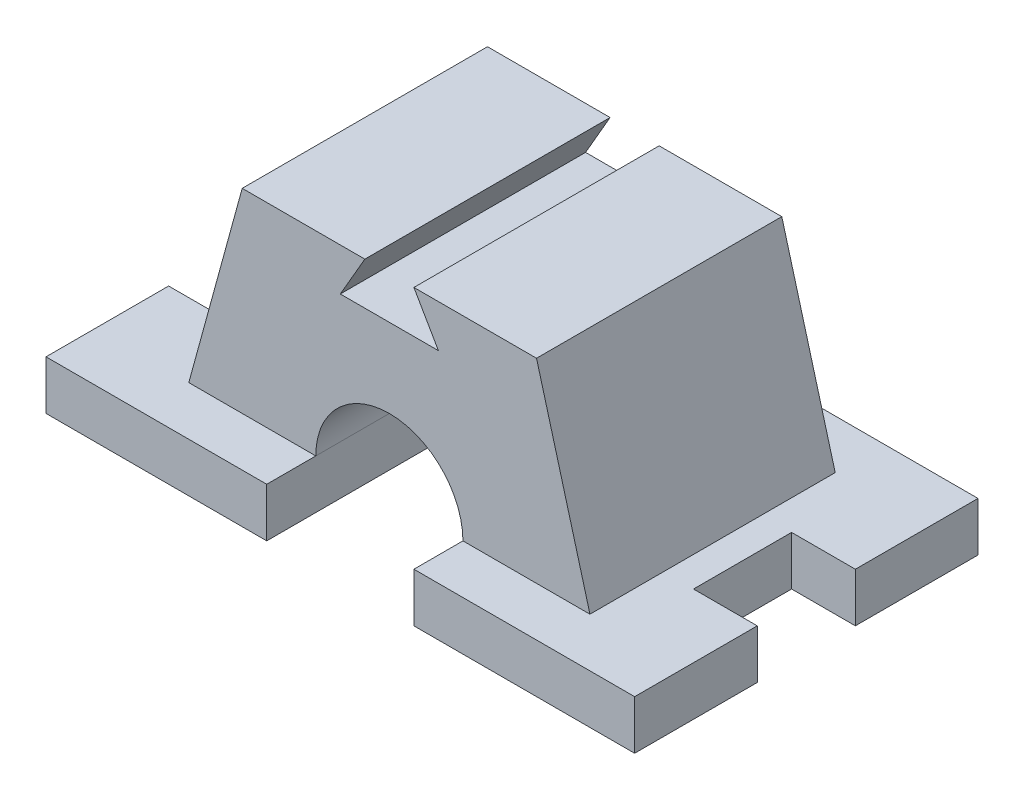
ISO-10303-21;
HEADER;
FILE_DESCRIPTION(('STEP AP214'),'2;1');
FILE_NAME('part.step','',(''),(''),'','','');
FILE_SCHEMA(('AUTOMOTIVE_DESIGN { 1 0 10303 214 1 1 1 1 }'));
ENDSEC;
DATA;
#1=APPLICATION_CONTEXT('core data for automotive mechanical design processes');
#2=APPLICATION_PROTOCOL_DEFINITION('international standard','automotive_design',2000,#1);
#3=PRODUCT_CONTEXT('',#1,'mechanical');
#4=PRODUCT('Part','Part','',(#3));
#5=PRODUCT_RELATED_PRODUCT_CATEGORY('part','',(#4));
#6=PRODUCT_DEFINITION_FORMATION('','',#4);
#7=PRODUCT_DEFINITION_CONTEXT('part definition',#1,'design');
#8=PRODUCT_DEFINITION('design','',#6,#7);
#9=PRODUCT_DEFINITION_SHAPE('','',#8);
#10=(LENGTH_UNIT() NAMED_UNIT(*) SI_UNIT(.MILLI.,.METRE.));
#11=(NAMED_UNIT(*) PLANE_ANGLE_UNIT() SI_UNIT($,.RADIAN.));
#12=(NAMED_UNIT(*) SI_UNIT($,.STERADIAN.) SOLID_ANGLE_UNIT());
#13=UNCERTAINTY_MEASURE_WITH_UNIT(LENGTH_MEASURE(1.E-05),#10,'distance_accuracy_value','');
#14=(GEOMETRIC_REPRESENTATION_CONTEXT(3) GLOBAL_UNCERTAINTY_ASSIGNED_CONTEXT((#13)) GLOBAL_UNIT_ASSIGNED_CONTEXT((#10,
#11,#12)) REPRESENTATION_CONTEXT('',''));
#15=CARTESIAN_POINT('',(0.,0.,0.));
#16=DIRECTION('',(0.,0.,1.));
#17=DIRECTION('',(1.,0.,0.));
#18=AXIS2_PLACEMENT_3D('',#15,#16,#17);
#19=CARTESIAN_POINT('',(42.8083356,10.,10.));
#20=DIRECTION('',(0.,0.,1.));
#21=DIRECTION('',(1.,0.,0.));
#22=AXIS2_PLACEMENT_3D('',#19,#20,#21);
#23=PLANE('',#22);
#24=DIRECTION('',(0.,-1.,0.));
#25=VECTOR('',#24,1.);
#26=CARTESIAN_POINT('',(46.9983356,0.,10.));
#27=LINE('',#26,#25);
#28=CARTESIAN_POINT('',(46.9983356,10.,10.));
#29=VERTEX_POINT('',#28);
#30=CARTESIAN_POINT('',(46.9983356,0.,10.));
#31=VERTEX_POINT('',#30);
#32=EDGE_CURVE('E59',#29,#31,#27,.T.);
#33=ORIENTED_EDGE('',*,*,#32,.F.);
#34=DIRECTION('',(-1.,0.,0.));
#35=VECTOR('',#34,1.);
#36=CARTESIAN_POINT('',(42.8083356,10.,10.));
#37=LINE('',#36,#35);
#38=CARTESIAN_POINT('',(60.,10.,10.));
#39=VERTEX_POINT('',#38);
#40=EDGE_CURVE('E227',#39,#29,#37,.T.);
#41=ORIENTED_EDGE('',*,*,#40,.F.);
#42=DIRECTION('',(0.,-1.,0.));
#43=VECTOR('',#42,1.);
#44=CARTESIAN_POINT('',(60.,10.,10.));
#45=LINE('',#44,#43);
#46=CARTESIAN_POINT('',(60.,0.,10.));
#47=VERTEX_POINT('',#46);
#48=EDGE_CURVE('E395',#39,#47,#45,.T.);
#49=ORIENTED_EDGE('',*,*,#48,.T.);
#50=DIRECTION('',(-1.,0.,0.));
#51=VECTOR('',#50,1.);
#52=CARTESIAN_POINT('',(42.8083356,0.,10.));
#53=LINE('',#52,#51);
#54=EDGE_CURVE('E64',#47,#31,#53,.T.);
#55=ORIENTED_EDGE('',*,*,#54,.T.);
#56=EDGE_LOOP('',(#33,#41,#49,#55));
#57=FACE_BOUND('',#56,.T.);
#58=ADVANCED_FACE('F43',(#57),#23,.F.);
#59=CARTESIAN_POINT('',(60.,10.,-10.));
#60=DIRECTION('',(0.,0.,-1.));
#61=DIRECTION('',(-1.,0.,0.));
#62=AXIS2_PLACEMENT_3D('',#59,#60,#61);
#63=PLANE('',#62);
#64=DIRECTION('',(0.,1.,0.));
#65=VECTOR('',#64,1.);
#66=CARTESIAN_POINT('',(46.9983356,10.,-10.));
#67=LINE('',#66,#65);
#68=CARTESIAN_POINT('',(46.9983356,0.,-10.));
#69=VERTEX_POINT('',#68);
#70=CARTESIAN_POINT('',(46.9983356,10.,-10.));
#71=VERTEX_POINT('',#70);
#72=EDGE_CURVE('E216',#69,#71,#67,.T.);
#73=ORIENTED_EDGE('',*,*,#72,.F.);
#74=DIRECTION('',(1.,0.,0.));
#75=VECTOR('',#74,1.);
#76=CARTESIAN_POINT('',(60.,0.,-10.));
#77=LINE('',#76,#75);
#78=CARTESIAN_POINT('',(60.,0.,-10.));
#79=VERTEX_POINT('',#78);
#80=EDGE_CURVE('E349',#69,#79,#77,.T.);
#81=ORIENTED_EDGE('',*,*,#80,.T.);
#82=DIRECTION('',(0.,-1.,0.));
#83=VECTOR('',#82,1.);
#84=CARTESIAN_POINT('',(60.,10.,-10.));
#85=LINE('',#84,#83);
#86=CARTESIAN_POINT('',(60.,10.,-10.));
#87=VERTEX_POINT('',#86);
#88=EDGE_CURVE('E225',#87,#79,#85,.T.);
#89=ORIENTED_EDGE('',*,*,#88,.F.);
#90=DIRECTION('',(1.,0.,0.));
#91=VECTOR('',#90,1.);
#92=CARTESIAN_POINT('',(60.,10.,-10.));
#93=LINE('',#92,#91);
#94=EDGE_CURVE('E217',#71,#87,#93,.T.);
#95=ORIENTED_EDGE('',*,*,#94,.F.);
#96=EDGE_LOOP('',(#73,#81,#89,#95));
#97=FACE_BOUND('',#96,.T.);
#98=ADVANCED_FACE('F219',(#97),#63,.F.);
#99=CARTESIAN_POINT('',(-60.,10.,-35.));
#100=DIRECTION('',(0.,0.,1.));
#101=DIRECTION('',(1.,0.,0.));
#102=AXIS2_PLACEMENT_3D('',#99,#100,#101);
#103=PLANE('',#102);
#104=DIRECTION('',(0.,-1.,0.));
#105=VECTOR('',#104,1.);
#106=CARTESIAN_POINT('',(-15.,10.,-35.));
#107=LINE('',#106,#105);
#108=CARTESIAN_POINT('',(-15.,10.,-35.));
#109=VERTEX_POINT('',#108);
#110=CARTESIAN_POINT('',(-15.,0.,-35.));
#111=VERTEX_POINT('',#110);
#112=EDGE_CURVE('E254',#109,#111,#107,.T.);
#113=ORIENTED_EDGE('',*,*,#112,.T.);
#114=DIRECTION('',(-1.,0.,0.));
#115=VECTOR('',#114,1.);
#116=CARTESIAN_POINT('',(-60.,0.,-35.));
#117=LINE('',#116,#115);
#118=CARTESIAN_POINT('',(-60.,0.,-35.));
#119=VERTEX_POINT('',#118);
#120=EDGE_CURVE('E369',#111,#119,#117,.T.);
#121=ORIENTED_EDGE('',*,*,#120,.T.);
#122=DIRECTION('',(0.,-1.,0.));
#123=VECTOR('',#122,1.);
#124=CARTESIAN_POINT('',(-60.,10.,-35.));
#125=LINE('',#124,#123);
#126=CARTESIAN_POINT('',(-60.,10.,-35.));
#127=VERTEX_POINT('',#126);
#128=EDGE_CURVE('E407',#127,#119,#125,.T.);
#129=ORIENTED_EDGE('',*,*,#128,.F.);
#130=DIRECTION('',(-1.,0.,0.));
#131=VECTOR('',#130,1.);
#132=CARTESIAN_POINT('',(-60.,10.,-35.));
#133=LINE('',#132,#131);
#134=EDGE_CURVE('E350',#109,#127,#133,.T.);
#135=ORIENTED_EDGE('',*,*,#134,.F.);
#136=EDGE_LOOP('',(#113,#121,#129,#135));
#137=FACE_BOUND('',#136,.T.);
#138=ADVANCED_FACE('F465',(#137),#103,.F.);
#139=DIRECTION('',(0.,1.,0.));
#140=VECTOR('',#139,1.);
#141=CARTESIAN_POINT('',(15.,10.,-35.));
#142=LINE('',#141,#140);
#143=CARTESIAN_POINT('',(15.,0.,-35.));
#144=VERTEX_POINT('',#143);
#145=CARTESIAN_POINT('',(15.,10.,-35.));
#146=VERTEX_POINT('',#145);
#147=EDGE_CURVE('E257',#144,#146,#142,.T.);
#148=ORIENTED_EDGE('',*,*,#147,.T.);
#149=CARTESIAN_POINT('',(60.,10.,-35.));
#150=VERTEX_POINT('',#149);
#151=EDGE_CURVE('E346',#150,#146,#133,.T.);
#152=ORIENTED_EDGE('',*,*,#151,.F.);
#153=DIRECTION('',(0.,-1.,0.));
#154=VECTOR('',#153,1.);
#155=CARTESIAN_POINT('',(60.,10.,-35.));
#156=LINE('',#155,#154);
#157=CARTESIAN_POINT('',(60.,0.,-35.));
#158=VERTEX_POINT('',#157);
#159=EDGE_CURVE('E51',#150,#158,#156,.T.);
#160=ORIENTED_EDGE('',*,*,#159,.T.);
#161=EDGE_CURVE('E371',#158,#144,#117,.T.);
#162=ORIENTED_EDGE('',*,*,#161,.T.);
#163=EDGE_LOOP('',(#148,#152,#160,#162));
#164=FACE_BOUND('',#163,.T.);
#165=ADVANCED_FACE('F412',(#164),#103,.F.);
#166=CARTESIAN_POINT('',(-60.,10.,35.));
#167=DIRECTION('',(0.,0.,-1.));
#168=DIRECTION('',(-1.,0.,0.));
#169=AXIS2_PLACEMENT_3D('',#166,#167,#168);
#170=PLANE('',#169);
#171=DIRECTION('',(0.,-1.,0.));
#172=VECTOR('',#171,1.);
#173=CARTESIAN_POINT('',(-15.,10.,35.));
#174=LINE('',#173,#172);
#175=CARTESIAN_POINT('',(-15.,10.,35.));
#176=VERTEX_POINT('',#175);
#177=CARTESIAN_POINT('',(-15.,0.,35.));
#178=VERTEX_POINT('',#177);
#179=EDGE_CURVE('E256',#176,#178,#174,.T.);
#180=ORIENTED_EDGE('',*,*,#179,.F.);
#181=DIRECTION('',(1.,0.,0.));
#182=VECTOR('',#181,1.);
#183=CARTESIAN_POINT('',(-60.,10.,35.));
#184=LINE('',#183,#182);
#185=CARTESIAN_POINT('',(-60.,10.,35.));
#186=VERTEX_POINT('',#185);
#187=EDGE_CURVE('E365',#186,#176,#184,.T.);
#188=ORIENTED_EDGE('',*,*,#187,.F.);
#189=DIRECTION('',(0.,-1.,0.));
#190=VECTOR('',#189,1.);
#191=CARTESIAN_POINT('',(-60.,10.,35.));
#192=LINE('',#191,#190);
#193=CARTESIAN_POINT('',(-60.,0.,35.));
#194=VERTEX_POINT('',#193);
#195=EDGE_CURVE('E400',#186,#194,#192,.T.);
#196=ORIENTED_EDGE('',*,*,#195,.T.);
#197=DIRECTION('',(1.,0.,0.));
#198=VECTOR('',#197,1.);
#199=CARTESIAN_POINT('',(-60.,0.,35.));
#200=LINE('',#199,#198);
#201=EDGE_CURVE('E381',#194,#178,#200,.T.);
#202=ORIENTED_EDGE('',*,*,#201,.T.);
#203=EDGE_LOOP('',(#180,#188,#196,#202));
#204=FACE_BOUND('',#203,.T.);
#205=ADVANCED_FACE('F448',(#204),#170,.F.);
#206=DIRECTION('',(0.,1.,0.));
#207=VECTOR('',#206,1.);
#208=CARTESIAN_POINT('',(15.,10.,35.));
#209=LINE('',#208,#207);
#210=CARTESIAN_POINT('',(15.,0.,35.));
#211=VERTEX_POINT('',#210);
#212=CARTESIAN_POINT('',(15.,10.,35.));
#213=VERTEX_POINT('',#212);
#214=EDGE_CURVE('E262',#211,#213,#209,.T.);
#215=ORIENTED_EDGE('',*,*,#214,.F.);
#216=CARTESIAN_POINT('',(60.,0.,35.));
#217=VERTEX_POINT('',#216);
#218=EDGE_CURVE('E384',#211,#217,#200,.T.);
#219=ORIENTED_EDGE('',*,*,#218,.T.);
#220=DIRECTION('',(0.,-1.,0.));
#221=VECTOR('',#220,1.);
#222=CARTESIAN_POINT('',(60.,10.,35.));
#223=LINE('',#222,#221);
#224=CARTESIAN_POINT('',(60.,10.,35.));
#225=VERTEX_POINT('',#224);
#226=EDGE_CURVE('E391',#225,#217,#223,.T.);
#227=ORIENTED_EDGE('',*,*,#226,.F.);
#228=EDGE_CURVE('E363',#213,#225,#184,.T.);
#229=ORIENTED_EDGE('',*,*,#228,.F.);
#230=EDGE_LOOP('',(#215,#219,#227,#229));
#231=FACE_BOUND('',#230,.T.);
#232=ADVANCED_FACE('F421',(#231),#170,.F.);
#233=CARTESIAN_POINT('',(0.,10.,0.));
#234=DIRECTION('',(0.,-1.,0.));
#235=DIRECTION('',(0.,0.,-1.));
#236=AXIS2_PLACEMENT_3D('',#233,#234,#235);
#237=PLANE('',#236);
#238=DIRECTION('',(1.,0.,0.));
#239=VECTOR('',#238,1.);
#240=CARTESIAN_POINT('',(-60.,10.,-10.));
#241=LINE('',#240,#239);
#242=CARTESIAN_POINT('',(-60.,10.,-10.));
#243=VERTEX_POINT('',#242);
#244=CARTESIAN_POINT('',(-47.,10.,-10.));
#245=VERTEX_POINT('',#244);
#246=EDGE_CURVE('E354',#243,#245,#241,.T.);
#247=ORIENTED_EDGE('',*,*,#246,.T.);
#248=DIRECTION('',(0.,0.,1.));
#249=VECTOR('',#248,1.);
#250=CARTESIAN_POINT('',(-47.,10.,10.));
#251=LINE('',#250,#249);
#252=CARTESIAN_POINT('',(-47.,10.,10.));
#253=VERTEX_POINT('',#252);
#254=EDGE_CURVE('E249',#245,#253,#251,.T.);
#255=ORIENTED_EDGE('',*,*,#254,.T.);
#256=DIRECTION('',(-1.,0.,0.));
#257=VECTOR('',#256,1.);
#258=CARTESIAN_POINT('',(-44.9850804,10.,10.));
#259=LINE('',#258,#257);
#260=CARTESIAN_POINT('',(-60.,10.,10.));
#261=VERTEX_POINT('',#260);
#262=EDGE_CURVE('E357',#253,#261,#259,.T.);
#263=ORIENTED_EDGE('',*,*,#262,.T.);
#264=DIRECTION('',(0.,0.,1.));
#265=VECTOR('',#264,1.);
#266=CARTESIAN_POINT('',(-60.,10.,35.));
#267=LINE('',#266,#265);
#268=EDGE_CURVE('E360',#261,#186,#267,.T.);
#269=ORIENTED_EDGE('',*,*,#268,.T.);
#270=ORIENTED_EDGE('',*,*,#187,.T.);
#271=DIRECTION('',(0.,0.,-1.));
#272=VECTOR('',#271,1.);
#273=CARTESIAN_POINT('',(-15.,10.,35.));
#274=LINE('',#273,#272);
#275=CARTESIAN_POINT('',(-15.,10.,25.));
#276=VERTEX_POINT('',#275);
#277=EDGE_CURVE('E271',#176,#276,#274,.T.);
#278=ORIENTED_EDGE('',*,*,#277,.T.);
#279=DIRECTION('',(1.,0.,0.));
#280=VECTOR('',#279,1.);
#281=CARTESIAN_POINT('',(0.,10.,25.));
#282=LINE('',#281,#280);
#283=CARTESIAN_POINT('',(-40.8896827024535,10.,25.));
#284=VERTEX_POINT('',#283);
#285=EDGE_CURVE('E284',#284,#276,#282,.T.);
#286=ORIENTED_EDGE('',*,*,#285,.F.);
#287=DIRECTION('',(0.,0.,1.));
#288=VECTOR('',#287,1.);
#289=CARTESIAN_POINT('',(-40.8896827024535,10.,-25.));
#290=LINE('',#289,#288);
#291=CARTESIAN_POINT('',(-40.8896827024535,10.,-25.));
#292=VERTEX_POINT('',#291);
#293=EDGE_CURVE('E330',#292,#284,#290,.T.);
#294=ORIENTED_EDGE('',*,*,#293,.F.);
#295=DIRECTION('',(1.,0.,0.));
#296=VECTOR('',#295,1.);
#297=CARTESIAN_POINT('',(0.,10.,-25.));
#298=LINE('',#297,#296);
#299=CARTESIAN_POINT('',(-15.,10.,-25.));
#300=VERTEX_POINT('',#299);
#301=EDGE_CURVE('E308',#292,#300,#298,.T.);
#302=ORIENTED_EDGE('',*,*,#301,.T.);
#303=EDGE_CURVE('E275',#300,#109,#274,.T.);
#304=ORIENTED_EDGE('',*,*,#303,.T.);
#305=ORIENTED_EDGE('',*,*,#134,.T.);
#306=DIRECTION('',(0.,0.,1.));
#307=VECTOR('',#306,1.);
#308=CARTESIAN_POINT('',(-60.,10.,-10.));
#309=LINE('',#308,#307);
#310=EDGE_CURVE('E355',#127,#243,#309,.T.);
#311=ORIENTED_EDGE('',*,*,#310,.T.);
#312=EDGE_LOOP('',(#247,#255,#263,#269,#270,#278,#286,#294,#302,#304,#305,#311));
#313=FACE_BOUND('',#312,.T.);
#314=ADVANCED_FACE('F442',(#313),#237,.F.);
#315=DIRECTION('',(0.,0.,-1.));
#316=VECTOR('',#315,1.);
#317=CARTESIAN_POINT('',(15.,10.,35.));
#318=LINE('',#317,#316);
#319=CARTESIAN_POINT('',(15.,10.,25.));
#320=VERTEX_POINT('',#319);
#321=EDGE_CURVE('E261',#213,#320,#318,.T.);
#322=ORIENTED_EDGE('',*,*,#321,.F.);
#323=ORIENTED_EDGE('',*,*,#228,.T.);
#324=DIRECTION('',(0.,0.,-1.));
#325=VECTOR('',#324,1.);
#326=CARTESIAN_POINT('',(60.,10.,35.));
#327=LINE('',#326,#325);
#328=EDGE_CURVE('E362',#225,#39,#327,.T.);
#329=ORIENTED_EDGE('',*,*,#328,.T.);
#330=ORIENTED_EDGE('',*,*,#40,.T.);
#331=DIRECTION('',(0.,0.,1.));
#332=VECTOR('',#331,1.);
#333=CARTESIAN_POINT('',(46.9983356,10.,10.));
#334=LINE('',#333,#332);
#335=EDGE_CURVE('E231',#71,#29,#334,.T.);
#336=ORIENTED_EDGE('',*,*,#335,.F.);
#337=ORIENTED_EDGE('',*,*,#94,.T.);
#338=DIRECTION('',(0.,0.,-1.));
#339=VECTOR('',#338,1.);
#340=CARTESIAN_POINT('',(60.,10.,-10.));
#341=LINE('',#340,#339);
#342=EDGE_CURVE('E343',#87,#150,#341,.T.);
#343=ORIENTED_EDGE('',*,*,#342,.T.);
#344=ORIENTED_EDGE('',*,*,#151,.T.);
#345=CARTESIAN_POINT('',(15.,10.,-25.));
#346=VERTEX_POINT('',#345);
#347=EDGE_CURVE('E264',#346,#146,#318,.T.);
#348=ORIENTED_EDGE('',*,*,#347,.F.);
#349=CARTESIAN_POINT('',(40.8896827024535,9.99999999999999,-25.));
#350=VERTEX_POINT('',#349);
#351=EDGE_CURVE('E310',#346,#350,#298,.T.);
#352=ORIENTED_EDGE('',*,*,#351,.T.);
#353=DIRECTION('',(0.,0.,1.));
#354=VECTOR('',#353,1.);
#355=CARTESIAN_POINT('',(40.8896827024535,9.99999999999999,-25.));
#356=LINE('',#355,#354);
#357=CARTESIAN_POINT('',(40.8896827024535,9.99999999999999,25.));
#358=VERTEX_POINT('',#357);
#359=EDGE_CURVE('E342',#350,#358,#356,.T.);
#360=ORIENTED_EDGE('',*,*,#359,.T.);
#361=EDGE_CURVE('E285',#320,#358,#282,.T.);
#362=ORIENTED_EDGE('',*,*,#361,.F.);
#363=EDGE_LOOP('',(#322,#323,#329,#330,#336,#337,#343,#344,#348,#352,#360,#362));
#364=FACE_BOUND('',#363,.T.);
#365=ADVANCED_FACE('F240',(#364),#237,.F.);
#366=CARTESIAN_POINT('',(0.,0.,0.));
#367=DIRECTION('',(0.,-1.,0.));
#368=DIRECTION('',(0.,0.,-1.));
#369=AXIS2_PLACEMENT_3D('',#366,#367,#368);
#370=PLANE('',#369);
#371=DIRECTION('',(0.,0.,-1.));
#372=VECTOR('',#371,1.);
#373=CARTESIAN_POINT('',(-47.,0.,-10.));
#374=LINE('',#373,#372);
#375=CARTESIAN_POINT('',(-47.,0.,10.));
#376=VERTEX_POINT('',#375);
#377=CARTESIAN_POINT('',(-47.,0.,-10.));
#378=VERTEX_POINT('',#377);
#379=EDGE_CURVE('E241',#376,#378,#374,.T.);
#380=ORIENTED_EDGE('',*,*,#379,.T.);
#381=DIRECTION('',(1.,0.,0.));
#382=VECTOR('',#381,1.);
#383=CARTESIAN_POINT('',(-60.,0.,-10.));
#384=LINE('',#383,#382);
#385=CARTESIAN_POINT('',(-60.,0.,-10.));
#386=VERTEX_POINT('',#385);
#387=EDGE_CURVE('E376',#386,#378,#384,.T.);
#388=ORIENTED_EDGE('',*,*,#387,.F.);
#389=DIRECTION('',(0.,0.,1.));
#390=VECTOR('',#389,1.);
#391=CARTESIAN_POINT('',(-60.,0.,-10.));
#392=LINE('',#391,#390);
#393=EDGE_CURVE('E372',#119,#386,#392,.T.);
#394=ORIENTED_EDGE('',*,*,#393,.F.);
#395=ORIENTED_EDGE('',*,*,#120,.F.);
#396=DIRECTION('',(0.,0.,-1.));
#397=VECTOR('',#396,1.);
#398=CARTESIAN_POINT('',(-15.,0.,35.));
#399=LINE('',#398,#397);
#400=EDGE_CURVE('E267',#178,#111,#399,.T.);
#401=ORIENTED_EDGE('',*,*,#400,.F.);
#402=ORIENTED_EDGE('',*,*,#201,.F.);
#403=DIRECTION('',(0.,0.,1.));
#404=VECTOR('',#403,1.);
#405=CARTESIAN_POINT('',(-60.,0.,35.));
#406=LINE('',#405,#404);
#407=CARTESIAN_POINT('',(-60.,0.,10.));
#408=VERTEX_POINT('',#407);
#409=EDGE_CURVE('E382',#408,#194,#406,.T.);
#410=ORIENTED_EDGE('',*,*,#409,.F.);
#411=DIRECTION('',(-1.,0.,0.));
#412=VECTOR('',#411,1.);
#413=CARTESIAN_POINT('',(-44.9850804,0.,10.));
#414=LINE('',#413,#412);
#415=EDGE_CURVE('E378',#376,#408,#414,.T.);
#416=ORIENTED_EDGE('',*,*,#415,.F.);
#417=EDGE_LOOP('',(#380,#388,#394,#395,#401,#402,#410,#416));
#418=FACE_BOUND('',#417,.T.);
#419=ADVANCED_FACE('F453',(#418),#370,.T.);
#420=ORIENTED_EDGE('',*,*,#218,.F.);
#421=DIRECTION('',(0.,0.,-1.));
#422=VECTOR('',#421,1.);
#423=CARTESIAN_POINT('',(15.,0.,35.));
#424=LINE('',#423,#422);
#425=EDGE_CURVE('E268',#211,#144,#424,.T.);
#426=ORIENTED_EDGE('',*,*,#425,.T.);
#427=ORIENTED_EDGE('',*,*,#161,.F.);
#428=DIRECTION('',(0.,0.,-1.));
#429=VECTOR('',#428,1.);
#430=CARTESIAN_POINT('',(60.,0.,-10.));
#431=LINE('',#430,#429);
#432=EDGE_CURVE('E328',#79,#158,#431,.T.);
#433=ORIENTED_EDGE('',*,*,#432,.F.);
#434=ORIENTED_EDGE('',*,*,#80,.F.);
#435=DIRECTION('',(0.,0.,-1.));
#436=VECTOR('',#435,1.);
#437=CARTESIAN_POINT('',(46.9983356,0.,-10.));
#438=LINE('',#437,#436);
#439=EDGE_CURVE('E234',#31,#69,#438,.T.);
#440=ORIENTED_EDGE('',*,*,#439,.F.);
#441=ORIENTED_EDGE('',*,*,#54,.F.);
#442=DIRECTION('',(0.,0.,-1.));
#443=VECTOR('',#442,1.);
#444=CARTESIAN_POINT('',(60.,0.,35.));
#445=LINE('',#444,#443);
#446=EDGE_CURVE('E390',#217,#47,#445,.T.);
#447=ORIENTED_EDGE('',*,*,#446,.F.);
#448=EDGE_LOOP('',(#420,#426,#427,#433,#434,#440,#441,#447));
#449=FACE_BOUND('',#448,.T.);
#450=ADVANCED_FACE('F418',(#449),#370,.T.);
#451=CARTESIAN_POINT('',(60.,10.,-10.));
#452=DIRECTION('',(-1.,0.,0.));
#453=DIRECTION('',(0.,0.,1.));
#454=AXIS2_PLACEMENT_3D('',#451,#452,#453);
#455=PLANE('',#454);
#456=ORIENTED_EDGE('',*,*,#432,.T.);
#457=ORIENTED_EDGE('',*,*,#159,.F.);
#458=ORIENTED_EDGE('',*,*,#342,.F.);
#459=ORIENTED_EDGE('',*,*,#88,.T.);
#460=EDGE_LOOP('',(#456,#457,#458,#459));
#461=FACE_BOUND('',#460,.T.);
#462=ADVANCED_FACE('F44',(#461),#455,.F.);
#463=CARTESIAN_POINT('',(-60.,10.,-10.));
#464=DIRECTION('',(1.,0.,0.));
#465=DIRECTION('',(0.,0.,-1.));
#466=AXIS2_PLACEMENT_3D('',#463,#464,#465);
#467=PLANE('',#466);
#468=ORIENTED_EDGE('',*,*,#393,.T.);
#469=DIRECTION('',(0.,-1.,0.));
#470=VECTOR('',#469,1.);
#471=CARTESIAN_POINT('',(-60.,10.,-10.));
#472=LINE('',#471,#470);
#473=EDGE_CURVE('E401',#243,#386,#472,.T.);
#474=ORIENTED_EDGE('',*,*,#473,.F.);
#475=ORIENTED_EDGE('',*,*,#310,.F.);
#476=ORIENTED_EDGE('',*,*,#128,.T.);
#477=EDGE_LOOP('',(#468,#474,#475,#476));
#478=FACE_BOUND('',#477,.T.);
#479=ADVANCED_FACE('F535',(#478),#467,.F.);
#480=CARTESIAN_POINT('',(-60.,10.,-10.));
#481=DIRECTION('',(0.,0.,-1.));
#482=DIRECTION('',(-1.,0.,0.));
#483=AXIS2_PLACEMENT_3D('',#480,#481,#482);
#484=PLANE('',#483);
#485=ORIENTED_EDGE('',*,*,#387,.T.);
#486=DIRECTION('',(0.,1.,0.));
#487=VECTOR('',#486,1.);
#488=CARTESIAN_POINT('',(-47.,10.,-10.));
#489=LINE('',#488,#487);
#490=EDGE_CURVE('E250',#378,#245,#489,.T.);
#491=ORIENTED_EDGE('',*,*,#490,.T.);
#492=ORIENTED_EDGE('',*,*,#246,.F.);
#493=ORIENTED_EDGE('',*,*,#473,.T.);
#494=EDGE_LOOP('',(#485,#491,#492,#493));
#495=FACE_BOUND('',#494,.T.);
#496=ADVANCED_FACE('F526',(#495),#484,.F.);
#497=CARTESIAN_POINT('',(-44.9850804,10.,10.));
#498=DIRECTION('',(0.,0.,1.));
#499=DIRECTION('',(1.,0.,0.));
#500=AXIS2_PLACEMENT_3D('',#497,#498,#499);
#501=PLANE('',#500);
#502=ORIENTED_EDGE('',*,*,#262,.F.);
#503=DIRECTION('',(0.,-1.,0.));
#504=VECTOR('',#503,1.);
#505=CARTESIAN_POINT('',(-47.,0.,10.));
#506=LINE('',#505,#504);
#507=EDGE_CURVE('E238',#253,#376,#506,.T.);
#508=ORIENTED_EDGE('',*,*,#507,.T.);
#509=ORIENTED_EDGE('',*,*,#415,.T.);
#510=DIRECTION('',(0.,-1.,0.));
#511=VECTOR('',#510,1.);
#512=CARTESIAN_POINT('',(-60.,10.,10.));
#513=LINE('',#512,#511);
#514=EDGE_CURVE('E397',#261,#408,#513,.T.);
#515=ORIENTED_EDGE('',*,*,#514,.F.);
#516=EDGE_LOOP('',(#502,#508,#509,#515));
#517=FACE_BOUND('',#516,.T.);
#518=ADVANCED_FACE('F521',(#517),#501,.F.);
#519=CARTESIAN_POINT('',(-60.,10.,35.));
#520=DIRECTION('',(1.,0.,0.));
#521=DIRECTION('',(0.,0.,-1.));
#522=AXIS2_PLACEMENT_3D('',#519,#520,#521);
#523=PLANE('',#522);
#524=ORIENTED_EDGE('',*,*,#409,.T.);
#525=ORIENTED_EDGE('',*,*,#195,.F.);
#526=ORIENTED_EDGE('',*,*,#268,.F.);
#527=ORIENTED_EDGE('',*,*,#514,.T.);
#528=EDGE_LOOP('',(#524,#525,#526,#527));
#529=FACE_BOUND('',#528,.T.);
#530=ADVANCED_FACE('F519',(#529),#523,.F.);
#531=CARTESIAN_POINT('',(60.,10.,35.));
#532=DIRECTION('',(-1.,0.,0.));
#533=DIRECTION('',(0.,0.,1.));
#534=AXIS2_PLACEMENT_3D('',#531,#532,#533);
#535=PLANE('',#534);
#536=ORIENTED_EDGE('',*,*,#446,.T.);
#537=ORIENTED_EDGE('',*,*,#48,.F.);
#538=ORIENTED_EDGE('',*,*,#328,.F.);
#539=ORIENTED_EDGE('',*,*,#226,.T.);
#540=EDGE_LOOP('',(#536,#537,#538,#539));
#541=FACE_BOUND('',#540,.T.);
#542=ADVANCED_FACE('F513',(#541),#535,.F.);
#543=CARTESIAN_POINT('',(-40.5833533821708,11.118159123164,-25.));
#544=DIRECTION('',(-0.964461725738686,0.264222594766526,0.));
#545=DIRECTION('',(-0.264222594766526,-0.964461725738686,0.));
#546=AXIS2_PLACEMENT_3D('',#543,#544,#545);
#547=PLANE('',#546);
#548=ORIENTED_EDGE('',*,*,#293,.T.);
#549=DIRECTION('',(-0.264222594766526,-0.964461725738686,0.));
#550=VECTOR('',#549,1.);
#551=CARTESIAN_POINT('',(-40.5833533821708,11.118159123164,25.));
#552=LINE('',#551,#550);
#553=CARTESIAN_POINT('',(-29.9999999999999,49.749371855331,25.));
#554=VERTEX_POINT('',#553);
#555=EDGE_CURVE('E276',#554,#284,#552,.T.);
#556=ORIENTED_EDGE('',*,*,#555,.F.);
#557=DIRECTION('',(0.,0.,1.));
#558=VECTOR('',#557,1.);
#559=CARTESIAN_POINT('',(-29.9999999999999,49.749371855331,-25.));
#560=LINE('',#559,#558);
#561=CARTESIAN_POINT('',(-29.9999999999999,49.749371855331,-25.));
#562=VERTEX_POINT('',#561);
#563=EDGE_CURVE('E329',#562,#554,#560,.T.);
#564=ORIENTED_EDGE('',*,*,#563,.F.);
#565=DIRECTION('',(-0.264222594766526,-0.964461725738686,0.));
#566=VECTOR('',#565,1.);
#567=CARTESIAN_POINT('',(-40.5833533821708,11.118159123164,-25.));
#568=LINE('',#567,#566);
#569=EDGE_CURVE('E302',#562,#292,#568,.T.);
#570=ORIENTED_EDGE('',*,*,#569,.T.);
#571=EDGE_LOOP('',(#548,#556,#564,#570));
#572=FACE_BOUND('',#571,.T.);
#573=ADVANCED_FACE('F496',(#572),#547,.T.);
#574=CARTESIAN_POINT('',(0.,49.749371855331,-25.));
#575=DIRECTION('',(0.,1.,0.));
#576=DIRECTION('',(0.,0.,1.));
#577=AXIS2_PLACEMENT_3D('',#574,#575,#576);
#578=PLANE('',#577);
#579=ORIENTED_EDGE('',*,*,#563,.T.);
#580=DIRECTION('',(-1.,0.,0.));
#581=VECTOR('',#580,1.);
#582=CARTESIAN_POINT('',(0.,49.749371855331,25.));
#583=LINE('',#582,#581);
#584=CARTESIAN_POINT('',(-4.99999999999992,49.749371855331,25.));
#585=VERTEX_POINT('',#584);
#586=EDGE_CURVE('E301',#585,#554,#583,.T.);
#587=ORIENTED_EDGE('',*,*,#586,.F.);
#588=DIRECTION('',(0.,0.,1.));
#589=VECTOR('',#588,1.);
#590=CARTESIAN_POINT('',(-4.99999999999992,49.749371855331,-25.));
#591=LINE('',#590,#589);
#592=CARTESIAN_POINT('',(-4.99999999999992,49.749371855331,-25.));
#593=VERTEX_POINT('',#592);
#594=EDGE_CURVE('E333',#593,#585,#591,.T.);
#595=ORIENTED_EDGE('',*,*,#594,.F.);
#596=DIRECTION('',(-1.,0.,0.));
#597=VECTOR('',#596,1.);
#598=CARTESIAN_POINT('',(0.,49.749371855331,-25.));
#599=LINE('',#598,#597);
#600=EDGE_CURVE('E321',#593,#562,#599,.T.);
#601=ORIENTED_EDGE('',*,*,#600,.T.);
#602=EDGE_LOOP('',(#579,#587,#595,#601));
#603=FACE_BOUND('',#602,.T.);
#604=ADVANCED_FACE('F494',(#603),#578,.T.);
#605=CARTESIAN_POINT('',(-25.2921099245176,14.602406473294,-25.));
#606=DIRECTION('',(0.866025403784436,-0.500000000000004,0.));
#607=DIRECTION('',(0.500000000000004,0.866025403784436,0.));
#608=AXIS2_PLACEMENT_3D('',#605,#606,#607);
#609=PLANE('',#608);
#610=ORIENTED_EDGE('',*,*,#594,.T.);
#611=DIRECTION('',(0.500000000000004,0.866025403784436,0.));
#612=VECTOR('',#611,1.);
#613=CARTESIAN_POINT('',(-25.2921099245176,14.602406473294,25.));
#614=LINE('',#613,#612);
#615=CARTESIAN_POINT('',(-10.,41.0891178174866,25.));
#616=VERTEX_POINT('',#615);
#617=EDGE_CURVE('E296',#616,#585,#614,.T.);
#618=ORIENTED_EDGE('',*,*,#617,.F.);
#619=DIRECTION('',(0.,0.,1.));
#620=VECTOR('',#619,1.);
#621=CARTESIAN_POINT('',(-10.,41.0891178174866,-25.));
#622=LINE('',#621,#620);
#623=CARTESIAN_POINT('',(-10.,41.0891178174866,-25.));
#624=VERTEX_POINT('',#623);
#625=EDGE_CURVE('E331',#624,#616,#622,.T.);
#626=ORIENTED_EDGE('',*,*,#625,.F.);
#627=DIRECTION('',(0.500000000000004,0.866025403784436,0.));
#628=VECTOR('',#627,1.);
#629=CARTESIAN_POINT('',(-25.2921099245176,14.602406473294,-25.));
#630=LINE('',#629,#628);
#631=EDGE_CURVE('E322',#624,#593,#630,.T.);
#632=ORIENTED_EDGE('',*,*,#631,.T.);
#633=EDGE_LOOP('',(#610,#618,#626,#632));
#634=FACE_BOUND('',#633,.T.);
#635=ADVANCED_FACE('F489',(#634),#609,.T.);
#636=CARTESIAN_POINT('',(0.,41.0891178174866,-25.));
#637=DIRECTION('',(0.,1.,0.));
#638=DIRECTION('',(-1.,0.,0.));
#639=AXIS2_PLACEMENT_3D('',#636,#637,#638);
#640=PLANE('',#639);
#641=ORIENTED_EDGE('',*,*,#625,.T.);
#642=DIRECTION('',(-1.,0.,0.));
#643=VECTOR('',#642,1.);
#644=CARTESIAN_POINT('',(0.,41.0891178174866,25.));
#645=LINE('',#644,#643);
#646=CARTESIAN_POINT('',(10.,41.0891178174866,25.));
#647=VERTEX_POINT('',#646);
#648=EDGE_CURVE('E294',#647,#616,#645,.T.);
#649=ORIENTED_EDGE('',*,*,#648,.F.);
#650=DIRECTION('',(0.,0.,1.));
#651=VECTOR('',#650,1.);
#652=CARTESIAN_POINT('',(10.,41.0891178174866,-25.));
#653=LINE('',#652,#651);
#654=CARTESIAN_POINT('',(10.,41.0891178174866,-25.));
#655=VERTEX_POINT('',#654);
#656=EDGE_CURVE('E332',#655,#647,#653,.T.);
#657=ORIENTED_EDGE('',*,*,#656,.F.);
#658=DIRECTION('',(-1.,0.,0.));
#659=VECTOR('',#658,1.);
#660=CARTESIAN_POINT('',(0.,41.0891178174866,-25.));
#661=LINE('',#660,#659);
#662=EDGE_CURVE('E319',#655,#624,#661,.T.);
#663=ORIENTED_EDGE('',*,*,#662,.T.);
#664=EDGE_LOOP('',(#641,#649,#657,#663));
#665=FACE_BOUND('',#664,.T.);
#666=ADVANCED_FACE('F500',(#665),#640,.T.);
#667=CARTESIAN_POINT('',(25.2921099245176,14.602406473294,-25.));
#668=DIRECTION('',(0.866025403784436,0.500000000000004,0.));
#669=DIRECTION('',(-0.500000000000004,0.866025403784436,0.));
#670=AXIS2_PLACEMENT_3D('',#667,#668,#669);
#671=PLANE('',#670);
#672=ORIENTED_EDGE('',*,*,#656,.T.);
#673=DIRECTION('',(-0.500000000000004,0.866025403784436,0.));
#674=VECTOR('',#673,1.);
#675=CARTESIAN_POINT('',(25.2921099245176,14.602406473294,25.));
#676=LINE('',#675,#674);
#677=CARTESIAN_POINT('',(4.99999999999992,49.749371855331,25.));
#678=VERTEX_POINT('',#677);
#679=EDGE_CURVE('E292',#647,#678,#676,.T.);
#680=ORIENTED_EDGE('',*,*,#679,.T.);
#681=DIRECTION('',(0.,0.,1.));
#682=VECTOR('',#681,1.);
#683=CARTESIAN_POINT('',(4.99999999999992,49.749371855331,-25.));
#684=LINE('',#683,#682);
#685=CARTESIAN_POINT('',(4.99999999999992,49.749371855331,-25.));
#686=VERTEX_POINT('',#685);
#687=EDGE_CURVE('E340',#686,#678,#684,.T.);
#688=ORIENTED_EDGE('',*,*,#687,.F.);
#689=DIRECTION('',(-0.500000000000004,0.866025403784436,0.));
#690=VECTOR('',#689,1.);
#691=CARTESIAN_POINT('',(25.2921099245176,14.602406473294,-25.));
#692=LINE('',#691,#690);
#693=EDGE_CURVE('E317',#655,#686,#692,.T.);
#694=ORIENTED_EDGE('',*,*,#693,.F.);
#695=EDGE_LOOP('',(#672,#680,#688,#694));
#696=FACE_BOUND('',#695,.T.);
#697=ADVANCED_FACE('F481',(#696),#671,.F.);
#698=CARTESIAN_POINT('',(0.,49.749371855331,-25.));
#699=DIRECTION('',(0.,-1.,0.));
#700=DIRECTION('',(0.,0.,-1.));
#701=AXIS2_PLACEMENT_3D('',#698,#699,#700);
#702=PLANE('',#701);
#703=ORIENTED_EDGE('',*,*,#687,.T.);
#704=DIRECTION('',(1.,0.,0.));
#705=VECTOR('',#704,1.);
#706=CARTESIAN_POINT('',(0.,49.749371855331,25.));
#707=LINE('',#706,#705);
#708=CARTESIAN_POINT('',(29.9999999999999,49.749371855331,25.));
#709=VERTEX_POINT('',#708);
#710=EDGE_CURVE('E289',#678,#709,#707,.T.);
#711=ORIENTED_EDGE('',*,*,#710,.T.);
#712=DIRECTION('',(0.,0.,1.));
#713=VECTOR('',#712,1.);
#714=CARTESIAN_POINT('',(29.9999999999999,49.749371855331,-25.));
#715=LINE('',#714,#713);
#716=CARTESIAN_POINT('',(29.9999999999999,49.749371855331,-25.));
#717=VERTEX_POINT('',#716);
#718=EDGE_CURVE('E339',#717,#709,#715,.T.);
#719=ORIENTED_EDGE('',*,*,#718,.F.);
#720=DIRECTION('',(1.,0.,0.));
#721=VECTOR('',#720,1.);
#722=CARTESIAN_POINT('',(0.,49.749371855331,-25.));
#723=LINE('',#722,#721);
#724=EDGE_CURVE('E313',#686,#717,#723,.T.);
#725=ORIENTED_EDGE('',*,*,#724,.F.);
#726=EDGE_LOOP('',(#703,#711,#719,#725));
#727=FACE_BOUND('',#726,.T.);
#728=ADVANCED_FACE('F479',(#727),#702,.F.);
#729=CARTESIAN_POINT('',(40.5833533821707,11.118159123164,-25.));
#730=DIRECTION('',(-0.964461725738686,-0.264222594766526,0.));
#731=DIRECTION('',(0.264222594766526,-0.964461725738686,0.));
#732=AXIS2_PLACEMENT_3D('',#729,#730,#731);
#733=PLANE('',#732);
#734=ORIENTED_EDGE('',*,*,#718,.T.);
#735=DIRECTION('',(0.264222594766526,-0.964461725738686,0.));
#736=VECTOR('',#735,1.);
#737=CARTESIAN_POINT('',(40.5833533821707,11.118159123164,25.));
#738=LINE('',#737,#736);
#739=EDGE_CURVE('E288',#709,#358,#738,.T.);
#740=ORIENTED_EDGE('',*,*,#739,.T.);
#741=ORIENTED_EDGE('',*,*,#359,.F.);
#742=DIRECTION('',(0.264222594766526,-0.964461725738686,0.));
#743=VECTOR('',#742,1.);
#744=CARTESIAN_POINT('',(40.5833533821707,11.118159123164,-25.));
#745=LINE('',#744,#743);
#746=EDGE_CURVE('E311',#717,#350,#745,.T.);
#747=ORIENTED_EDGE('',*,*,#746,.F.);
#748=EDGE_LOOP('',(#734,#740,#741,#747));
#749=FACE_BOUND('',#748,.T.);
#750=ADVANCED_FACE('F474',(#749),#733,.F.);
#751=CARTESIAN_POINT('',(0.,0.,-25.));
#752=DIRECTION('',(0.,0.,1.));
#753=DIRECTION('',(1.,0.,0.));
#754=AXIS2_PLACEMENT_3D('',#751,#752,#753);
#755=PLANE('',#754);
#756=CARTESIAN_POINT('',(0.,10.,-25.));
#757=DIRECTION('',(0.,0.,1.));
#758=DIRECTION('',(1.,0.,0.));
#759=AXIS2_PLACEMENT_3D('',#756,#757,#758);
#760=CIRCLE('',#759,15.);
#761=EDGE_CURVE('E277',#300,#346,#760,.F.);
#762=ORIENTED_EDGE('',*,*,#761,.F.);
#763=ORIENTED_EDGE('',*,*,#301,.F.);
#764=ORIENTED_EDGE('',*,*,#569,.F.);
#765=ORIENTED_EDGE('',*,*,#600,.F.);
#766=ORIENTED_EDGE('',*,*,#631,.F.);
#767=ORIENTED_EDGE('',*,*,#662,.F.);
#768=ORIENTED_EDGE('',*,*,#693,.T.);
#769=ORIENTED_EDGE('',*,*,#724,.T.);
#770=ORIENTED_EDGE('',*,*,#746,.T.);
#771=ORIENTED_EDGE('',*,*,#351,.F.);
#772=EDGE_LOOP('',(#762,#763,#764,#765,#766,#767,#768,#769,#770,#771));
#773=FACE_BOUND('',#772,.T.);
#774=ADVANCED_FACE('F466',(#773),#755,.F.);
#775=CARTESIAN_POINT('',(0.,0.,25.));
#776=DIRECTION('',(0.,0.,1.));
#777=DIRECTION('',(1.,0.,0.));
#778=AXIS2_PLACEMENT_3D('',#775,#776,#777);
#779=PLANE('',#778);
#780=ORIENTED_EDGE('',*,*,#285,.T.);
#781=CARTESIAN_POINT('',(0.,10.,25.));
#782=DIRECTION('',(0.,0.,1.));
#783=DIRECTION('',(1.,0.,0.));
#784=AXIS2_PLACEMENT_3D('',#781,#782,#783);
#785=CIRCLE('',#784,15.);
#786=EDGE_CURVE('E11',#276,#320,#785,.F.);
#787=ORIENTED_EDGE('',*,*,#786,.T.);
#788=ORIENTED_EDGE('',*,*,#361,.T.);
#789=ORIENTED_EDGE('',*,*,#739,.F.);
#790=ORIENTED_EDGE('',*,*,#710,.F.);
#791=ORIENTED_EDGE('',*,*,#679,.F.);
#792=ORIENTED_EDGE('',*,*,#648,.T.);
#793=ORIENTED_EDGE('',*,*,#617,.T.);
#794=ORIENTED_EDGE('',*,*,#586,.T.);
#795=ORIENTED_EDGE('',*,*,#555,.T.);
#796=EDGE_LOOP('',(#780,#787,#788,#789,#790,#791,#792,#793,#794,#795));
#797=FACE_BOUND('',#796,.T.);
#798=ADVANCED_FACE('F440',(#797),#779,.T.);
#799=CARTESIAN_POINT('',(0.,10.,35.));
#800=DIRECTION('',(0.,0.,-1.));
#801=DIRECTION('',(-1.,0.,0.));
#802=AXIS2_PLACEMENT_3D('',#799,#800,#801);
#803=CYLINDRICAL_SURFACE('',#802,15.);
#804=ORIENTED_EDGE('',*,*,#761,.T.);
#805=EDGE_CURVE('E270',#320,#346,#318,.T.);
#806=ORIENTED_EDGE('',*,*,#805,.F.);
#807=ORIENTED_EDGE('',*,*,#786,.F.);
#808=EDGE_CURVE('E280',#276,#300,#274,.T.);
#809=ORIENTED_EDGE('',*,*,#808,.T.);
#810=EDGE_LOOP('',(#804,#806,#807,#809));
#811=FACE_BOUND('',#810,.T.);
#812=ADVANCED_FACE('F435',(#811),#803,.F.);
#813=CARTESIAN_POINT('',(-15.,10.,35.));
#814=DIRECTION('',(1.,0.,0.));
#815=DIRECTION('',(0.,0.,-1.));
#816=AXIS2_PLACEMENT_3D('',#813,#814,#815);
#817=PLANE('',#816);
#818=ORIENTED_EDGE('',*,*,#277,.F.);
#819=ORIENTED_EDGE('',*,*,#179,.T.);
#820=ORIENTED_EDGE('',*,*,#400,.T.);
#821=ORIENTED_EDGE('',*,*,#112,.F.);
#822=ORIENTED_EDGE('',*,*,#303,.F.);
#823=ORIENTED_EDGE('',*,*,#808,.F.);
#824=EDGE_LOOP('',(#818,#819,#820,#821,#822,#823));
#825=FACE_BOUND('',#824,.T.);
#826=ADVANCED_FACE('F450',(#825),#817,.T.);
#827=CARTESIAN_POINT('',(15.,10.,35.));
#828=DIRECTION('',(-1.,0.,0.));
#829=DIRECTION('',(0.,-1.,0.));
#830=AXIS2_PLACEMENT_3D('',#827,#828,#829);
#831=PLANE('',#830);
#832=ORIENTED_EDGE('',*,*,#425,.F.);
#833=ORIENTED_EDGE('',*,*,#214,.T.);
#834=ORIENTED_EDGE('',*,*,#321,.T.);
#835=ORIENTED_EDGE('',*,*,#805,.T.);
#836=ORIENTED_EDGE('',*,*,#347,.T.);
#837=ORIENTED_EDGE('',*,*,#147,.F.);
#838=EDGE_LOOP('',(#832,#833,#834,#835,#836,#837));
#839=FACE_BOUND('',#838,.T.);
#840=ADVANCED_FACE('F417',(#839),#831,.T.);
#841=CARTESIAN_POINT('',(-47.,0.,0.));
#842=DIRECTION('',(-1.,0.,0.));
#843=DIRECTION('',(0.,0.,1.));
#844=AXIS2_PLACEMENT_3D('',#841,#842,#843);
#845=PLANE('',#844);
#846=ORIENTED_EDGE('',*,*,#507,.F.);
#847=ORIENTED_EDGE('',*,*,#254,.F.);
#848=ORIENTED_EDGE('',*,*,#490,.F.);
#849=ORIENTED_EDGE('',*,*,#379,.F.);
#850=EDGE_LOOP('',(#846,#847,#848,#849));
#851=FACE_BOUND('',#850,.T.);
#852=ADVANCED_FACE('F586',(#851),#845,.T.);
#853=CARTESIAN_POINT('',(46.9983356,0.,0.));
#854=DIRECTION('',(-1.,0.,0.));
#855=DIRECTION('',(0.,0.,1.));
#856=AXIS2_PLACEMENT_3D('',#853,#854,#855);
#857=PLANE('',#856);
#858=ORIENTED_EDGE('',*,*,#32,.T.);
#859=ORIENTED_EDGE('',*,*,#439,.T.);
#860=ORIENTED_EDGE('',*,*,#72,.T.);
#861=ORIENTED_EDGE('',*,*,#335,.T.);
#862=EDGE_LOOP('',(#858,#859,#860,#861));
#863=FACE_BOUND('',#862,.T.);
#864=ADVANCED_FACE('F235',(#863),#857,.F.);
#865=CLOSED_SHELL('',(#58,#98,#138,#165,#205,#232,#314,#365,#419,#450,#462,#479,#496,#518,#530,
#542,#573,#604,#635,#666,#697,#728,#750,#774,#798,#812,#826,#840,#852,#864));
#866=MANIFOLD_SOLID_BREP('B2',#865);
#867=ADVANCED_BREP_SHAPE_REPRESENTATION('',(#18,#866),#14);
#868=SHAPE_DEFINITION_REPRESENTATION(#9,#867);
ENDSEC;
END-ISO-10303-21;
